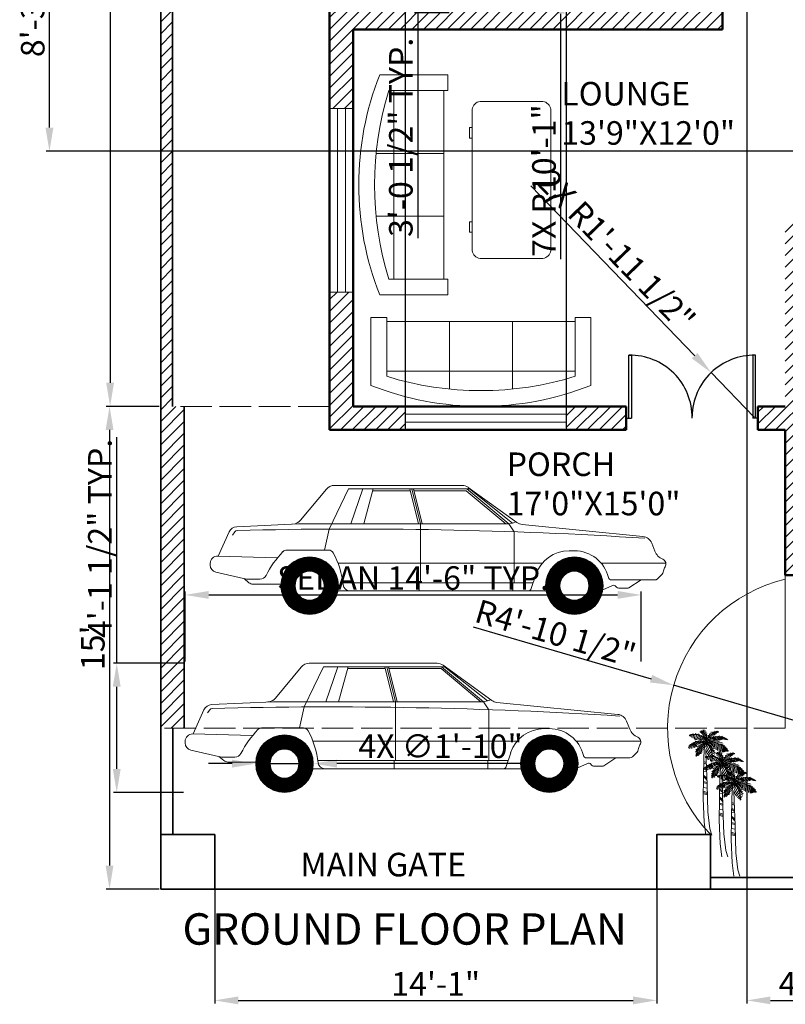
# Model space of a CAD drawing. Units: inches. Extents: x 36184 to 36805, y 18177 to 19069.
# Tile 1 of 5: x 36191 to 36484, y 18183 to 18560. Entities that reach past the tile are written whole.
import ezdxf

# ---------------------------------------------------------------- set-up
doc = ezdxf.new("R2010")
doc.units = ezdxf.units.IN
doc.linetypes.add('ACAD_ISO02W100', pattern=[15, 12, -3])
for name, color, linetype, lineweight in [('A-ANNO-DIMS', 2, 'Continuous', 18), ('A-ANNO-TEXT', 7, 'Continuous', 18), ('A-AREA-IDEN', 7, 'Continuous', 25), ('A-DOOR', 4, 'Continuous', 25), ('A-FURN', 8, 'Continuous', 18), ('A-GLAZ', 4, 'Continuous', 18), ('A-ROOF-OVHD', 8, 'ACAD_ISO02W100', 18), ('A-WALL', 7, 'Continuous', 50), ('C-PRKG-VEHS', 8, 'Continuous', 13), ('C-PROP', 7, 'Continuous', 35), ('L-HRDS', 8, 'Continuous', 18), ('L-PLNT', 94, 'Continuous', 13), ('L-SITE-GATE', 7, 'Continuous', 35), ('L-SITE-WALL', 7, 'Continuous', 35), ('L-WALL-PATT', 7, 'Continuous', 13)]:
    doc.layers.add(name, color=color, linetype=linetype, lineweight=lineweight)
doc.layers.add('A-WALL-PATT', color=244, linetype='Continuous', lineweight=13, true_color=0x991b1e)
doc.styles.get("Standard").update_dxf_attribs({"font": 'arial.ttf'})
doc.dimstyles.new('ISO-25', dxfattribs={"dimtxt": 9, "dimasz": 9, "dimexe": 1.25, "dimexo": 0.625, "dimtad": 1, "dimdec": 1, "dimrnd": 9, "dimlunit": 3, "dimtxsty": 'Standard', "dimcen": 2.5, "dimadec": 0, "dimazin": 0, "dimtfac": 1, "dimtdec": 1, "dimtmove": 0, "dimatfit": 3, "dimfxl": 1, "dimarcsym": 0})

# ---------------------------------------------------------------- blocks, each defined once
blk = doc.blocks.new('Car - sedan  side')
for p, q in [((-77.81, 49.34), (-126.58, 49.34)), ((-139.53, 35.99), (-129.64, 47.91)), ((-128.57, 32.64), (-121.22, 48.02)), ((-74.7, 48.02), (-121.22, 48.02)), ((-120.32, 34.67), (-115.67, 48.02)), ((-115.4, 34.67), (-111.74, 48.02)), ((-97.55, 47.3), (-111.94, 47.3)), ((-94.41, 34.67), (-97.73, 48.02)), ((-93.72, 34.67), (-97.04, 48.02)), ((-93.03, 34.67), (-96.34, 48.02)), ((-76.26, 47.3), (-96.16, 47.3)), ((-61.08, 34.66), (-76.26, 47.3)), ((-60.02, 34.65), (-76.07, 48.02)), ((-56.87, 35.13), (-75.48, 48.59)), ((-58.54, 34.93), (-74.99, 48.02)), ((-140.23, 34.67), (-163.88, 33.56)), ((-62.28, 34.67), (-140.23, 34.67)), ((-93.72, 19.62), (-93.72, 34.67)), ((-62.28, 34.67), (-60.02, 34.65)), ((-60.02, 34.65), (-58.54, 34.93)), ((-57.97, 31.61), (-60.02, 34.65)), ((-57.21, 35.38), (-58.54, 34.93)), ((-54.93, 34.4), (-8.75, 29.8)), ((-170.93, 22.32), (-166.81, 31.56)), ((-164.57, 31.6), (-165.48, 30.35)), ((-130.39, 24.63), (-128.57, 32.64)), ((-57.97, 19.62), (-57.97, 31.61)), ((-4.21, 24.18), (-5.42, 27.27)), ((-128.78, 24.63), (-144.79, 24.63)), ((-36.97, 24.38), (-34.94, 24.38)), ((-174, 19.51), (-174, 18.91)), ((-148.26, 21.7), (-171.11, 22.33)), ((-47.2, 19.62), (-125.23, 19.62)), ((-93.72, 12.14), (-93.72, 19.62)), ((-57.97, 12.14), (-57.97, 19.62)), ((0, 19.62), (-24.7, 19.62)), ((-160.12, 13.48), (-171.81, 16.16)), ((-51.4, 9.89), (-49.69, 15.14)), ((-159.22, 12.14), (-161.08, 13.7)), ((-155.01, 13.48), (-160.12, 13.48)), ((-147.03, 11.6), (-157.73, 11.6)), ((-50.67, 12.14), (-123.32, 12.14)), ((-94.21, 9.03), (-94.21, 12.14)), ((-58.39, 9.03), (-58.39, 12.14)), ((-4.23, 13.19), (-20.72, 13.19)), ((-9.5, 13.19), (-14.1, 10.2)), ((-3.22, 13.59), (-1.77, 14.97)), ((-120.62, 9.03), (-125.23, 9.03)), ((-45.76, 9.03), (-120.62, 9.03)), ((-20.36, 11.06), (-24.06, 9.44)), ((-18.83, 10.42), (-19.11, 10.76)), ((-14.68, 10.03), (-18.01, 10.03))]:
    blk.add_line(p, q)
at = {"const_width": 5.49}
for points in [[(-127.8, 11, -1), (-144.3, 11, -1)], [(-26.69, 11, -1), (-43.19, 11, -1)]]:
    blk.add_lwpolyline(points, format="xyb", close=True, dxfattribs=at)
for centre, radius in [((-136.05, 11), 11), ((-34.94, 11), 11), ((-136.05, 11), 5.51), ((-34.94, 11), 5.51)]:
    blk.add_circle(centre, radius)
for centre, radius, start, end in [((-126.58, 45.38), 3.97, 90, 140.3029), ((-77.81, 45.38), 3.97, 54.135, 90), ((-142.58, 38.53), 3.97, 272.6827, 320.3029), ((-54.54, 38.35), 3.97, 234.135, 264.3123), ((-163.72, 30.18), 3.38, 92.6827, 155.9736), ((-163.62, 30.91), 1.17, 91.491, 143.9553), ((-118.51, -1702.12), 1734.79, 86.34698, 91.49105), ((-9.15, 25.82), 4, 21.3107, 84.3123), ((-118.09, -2.78), 38.85, 136.3964, 152.9097), ((-144.79, 22.64), 1.98, 90, 136.3964), ((-128.78, 22.64), 1.98, 28.1371, 90), ((-157.14, 7.48), 34.14, 6.5135, 28.1371), ((-36.97, 11), 13.38, 90, 161.9732), ((-34.94, 11), 13.38, 13.5864, 90), ((0.9, 26.18), 5.49, 201.3107, 247.7048), ((-171.18, 19.51), 2.82, 88.4193, 180), ((-171.18, 18.91), 2.82, 180, 257.0905), ((-1.92, 19.3), 1.94, 325.3744, 67.7048), ((-3.82, 17.12), 2.96, 313.7173, 352.3839), ((2.46, 16.28), 3.37, 145.3744, 172.3839), ((-157.73, 13.93), 2.32, 230.1291, 270), ((-155.01, 16.1), 2.62, 270, 332.9097), ((-120.62, 11.65), 2.62, 186.5135, 270), ((-20.72, 14.43), 1.24, 193.5864, 270), ((-4.23, 14.65), 1.46, 270, 313.7173), ((-52.58, 10.27), 1.24, 270, 341.9732), ((-19.93, 10.09), 1.06, 39.301, 113.7159), ((-18.01, 11.09), 1.06, 219.301, 270), ((-14.68, 11.09), 1.06, 270, 303.047)]:
    blk.add_arc(centre, radius, start, end)
blk = doc.blocks.new('Tree - palm elevation')
for p, q in [((-29.729, 190.759), (-31.469, 191.255)), ((-30.309, 190.512), (-30.695, 189.025)), ((-25.283, 191.751), (-29.342, 192.246)), ((-28.763, 190.759), (-28.763, 188.281)), ((-26.443, 191.503), (-26.636, 186.051)), ((-20.064, 191.751), (-25.863, 193.238)), ((-23.737, 191.751), (-24.51, 185.06)), ((-21.031, 191.998), (-21.804, 183.325)), ((-15.232, 191.255), (-20.644, 193.981)), ((-17.551, 191.503), (-20.451, 181.343)), ((-14.265, 190.759), (-18.131, 182.086)), ((-9.433, 189.025), (-15.618, 193.238)), ((-11.753, 189.768), (-15.425, 182.83)), ((-6.727, 197.202), (-11.366, 197.45)), ((-3.441, 194.477), (-10.013, 195.716)), ((-1.894, 192.494), (-9.24, 193.733)), ((-6.147, 186.299), (-9.24, 190.264)), ((-7.5, 199.68), (-7.5, 197.946)), ((-0.541, 189.52), (-7.307, 192.494)), ((-5.76, 190.016), (0.618, 185.308)), ((-5.567, 196.707), (-4.987, 201.167)), ((-4.407, 195.716), (-3.247, 200.672)), ((-2.474, 193.733), (-1.315, 199.433)), ((-1.121, 190.759), (0.232, 196.955)), ((0.038, 188.281), (1.778, 193.981)), ((1.005, 185.803), (2.358, 190.759)), ((4.098, 185.06), (4.678, 190.512)), ((5.837, 187.786), (7.577, 194.229)), ((6.997, 188.529), (12.216, 187.786)), ((8.544, 190.512), (13.763, 189.52)), ((9.317, 191.255), (10.283, 196.955)), ((11.25, 192.494), (15.889, 190.512)), ((11.829, 192.99), (13.182, 197.45)), ((13.956, 194.229), (14.729, 196.955)), ((14.536, 193.981), (17.242, 191.255)), ((15.116, 194.477), (17.822, 198.689)), ((15.695, 186.299), (19.368, 188.777)), ((16.082, 194.972), (17.822, 192.494)), ((18.015, 195.716), (20.914, 198.689)), ((18.015, 195.468), (18.981, 192.494)), ((19.368, 196.459), (19.948, 193.733)), ((19.368, 187.29), (26.133, 189.768)), ((20.914, 196.459), (21.301, 194.972)), ((21.301, 196.459), (22.847, 198.441)), ((22.074, 196.707), (23.427, 195.716)), ((23.234, 196.707), (23.62, 197.698)), ((24.78, 187.538), (31.546, 188.777)), ((-28.956, 172.174), (-32.435, 170.192)), ((-31.082, 169.944), (-32.435, 169.2)), ((-27.409, 173.413), (-30.695, 172.67)), ((-29.922, 170.687), (-27.989, 165.235)), ((-25.09, 175.148), (-28.376, 174.404)), ((-27.989, 172.422), (-26.056, 166.227)), ((-26.829, 173.661), (-23.544, 167.218)), ((-25.476, 174.652), (-21.224, 167.466)), ((-21.031, 177.626), (-24.897, 176.387)), ((-24.317, 175.891), (-18.711, 168.457)), ((-22.191, 176.635), (-16.391, 169.448)), ((-15.618, 179.36), (-20.644, 178.617)), ((-20.064, 177.626), (-15.812, 172.67)), ((-17.358, 178.617), (-13.299, 173.661)), ((-8.466, 171.678), (-16.585, 167.713)), ((-15.038, 179.36), (-10.786, 174.404)), ((-4.214, 175.148), (-14.072, 170.935)), ((-8.08, 188.034), (-12.912, 182.83)), ((-12.332, 180.104), (-9.433, 175.643)), ((-4.987, 185.803), (-10.979, 182.086)), ((-10.206, 180.104), (-8.08, 175.891)), ((-8.853, 170.935), (-7.113, 160.527)), ((-1.701, 176.882), (-8.66, 175.396)), ((-8.273, 180.104), (-6.147, 176.635)), ((-3.247, 183.821), (-8.08, 181.838)), ((-6.92, 172.917), (-5.374, 163.253)), ((-6.34, 179.608), (-4.6, 177.13)), ((-5.76, 188.034), (-1.508, 182.582)), ((-1.315, 181.591), (-5.374, 181.095)), ((-4.6, 174.9), (-4.021, 166.722)), ((-4.021, 179.36), (-2.861, 177.378)), ((-2.668, 185.803), (1.198, 181.343)), ((-2.668, 176.387), (-2.376, 170.594)), ((-0.348, 180.352), (-1.894, 180.104)), ((-0.928, 176.882), (-1.508, 173.909)), ((2.551, 175.891), (-0.928, 171.431)), ((3.711, 174.404), (-0.541, 167.961)), ((5.257, 171.926), (-0.155, 163.005)), ((1.585, 177.13), (0.038, 174.652)), ((1.005, 182.582), (2.938, 186.547)), ((1.585, 177.13), (6.61, 176.139)), ((2.938, 182.582), (6.61, 183.821)), ((2.938, 175.891), (8.737, 173.413)), ((4.098, 180.847), (8.35, 179.608)), ((4.291, 173.909), (12.216, 168.953)), ((4.871, 186.051), (10.09, 186.547)), ((4.871, 181.591), (8.544, 184.812)), ((5.644, 181.838), (13.569, 178.865)), ((6.224, 178.121), (8.157, 175.148)), ((6.417, 170.439), (14.729, 164.492)), ((7.384, 178.369), (10.476, 179.36)), ((7.77, 183.325), (16.082, 179.856)), ((8.157, 178.121), (10.476, 172.422)), ((9.51, 184.317), (15.502, 188.034)), ((10.476, 177.874), (12.796, 169.696)), ((11.25, 184.812), (17.628, 180.352)), ((11.829, 177.874), (18.015, 179.113)), ((13.182, 177.874), (14.729, 166.97)), ((14.536, 185.803), (19.948, 180.847)), ((15.889, 177.13), (16.855, 164.492)), ((17.242, 186.547), (23.041, 180.599)), ((18.015, 177.13), (26.133, 179.113)), ((18.981, 175.891), (19.561, 163.005)), ((20.721, 187.042), (25.167, 181.343)), ((20.914, 175.891), (30.966, 176.635)), ((21.688, 175.396), (22.074, 161.518)), ((23.814, 187.29), (26.907, 181.343)), ((23.814, 174.404), (25.554, 160.279)), ((25.554, 173.661), (33.285, 173.661)), ((26.133, 187.29), (29.419, 181.838)), ((26.52, 173.165), (28.066, 159.784)), ((28.066, 187.29), (30.966, 182.582)), ((28.839, 172.174), (36.378, 170.687)), ((29.226, 171.926), (30.966, 158.545)), ((29.806, 186.795), (32.319, 183.078)), ((29.999, 186.795), (33.092, 187.29)), ((30.966, 170.687), (38.891, 167.713)), ((32.126, 169.696), (32.512, 158.545)), ((32.512, 186.299), (35.218, 186.299)), ((33.479, 186.051), (34.445, 182.83)), ((35.605, 185.556), (37.151, 185.308)), ((35.798, 185.308), (36.958, 181.591)), ((38.118, 184.317), (38.504, 181.838)), ((39.857, 182.83), (40.244, 181.591)), ((-32.628, 167.961), (-33.208, 167.961)), ((-32.628, 167.713), (-32.435, 165.979)), ((-31.662, 168.705), (-31.082, 165.483)), ((-14.265, 164.244), (-19.678, 158.049)), ((-16.005, 160.031), (-19.484, 154.084)), ((-18.131, 153.589), (-19.484, 151.606)), ((-12.139, 167.961), (-19.098, 162.014)), ((-17.938, 152.597), (-16.972, 151.111)), ((-17.358, 155.819), (-14.845, 151.358)), ((-16.585, 158.545), (-13.106, 152.35)), ((-15.618, 160.775), (-12.332, 154.332)), ((-14.265, 163.749), (-10.786, 154.828)), ((-12.719, 166.722), (-9.046, 154.828)), ((-10.979, 168.457), (-7.887, 157.801)), ((7.384, 168.705), (0.812, 157.553)), ((9.317, 164.244), (2.358, 154.332)), ((10.863, 159.784), (4.484, 152.35)), ((11.829, 155.075), (6.804, 150.119)), ((8.544, 165.979), (16.662, 160.527)), ((12.603, 151.111), (8.544, 148.385)), ((10.09, 162.51), (17.435, 157.058)), ((11.443, 157.553), (16.855, 154.332)), ((12.216, 153.093), (16.082, 151.606)), ((34.058, 168.705), (34.445, 158.545)), ((35.412, 167.713), (41.404, 164.988)), ((36.378, 166.474), (35.605, 158.792)), ((37.731, 165.235), (36.958, 159.288)), ((37.924, 165.235), (41.404, 163.749)), ((38.504, 164.492), (38.504, 159.536)), ((39.664, 163.253), (42.37, 161.766)), ((39.857, 162.757), (39.857, 160.031)), ((40.824, 161.766), (41.21, 160.031)), ((41.21, 161.518), (42.757, 160.279)), ((-4.081, 140.645), (0.753, 138.261)), ((-4.081, 137.547), (0.753, 135.163)), ((12.216, 148.137), (10.09, 147.393)), ((12.409, 145.659), (11.056, 145.659)), ((12.409, 146.898), (13.763, 146.402)), ((12.603, 149.872), (15.116, 149.128)), ((-4.267, 114.428), (1.682, 108.708)), ((-4.081, 129.205), (1.124, 126.821)), ((-4.081, 127.298), (1.31, 123.246)), ((-4.081, 121.578), (1.31, 120.863)), ((-4.639, 102.273), (1.868, 100.604)), ((-4.453, 112.283), (1.682, 105.133)), ((-4.453, 99.651), (2.24, 98.459)), ((-4.825, 83.921), (2.612, 81.061)), ((-4.639, 81.299), (2.797, 78.916)), ((-4.639, 78.916), (2.797, 76.771)), ((-4.453, 91.071), (2.426, 89.641))]:
    blk.add_line(p, q)
for points in [[(-2.363, 170.553), (-3.88, 148.505), (-4.988, 69.634), (-3.325, 24.869), (0, 0)], [(-0.116, 162.848), (0.554, 143.532), (2.217, 96.635), (3.88, 44.054), (7.76, 12.079), (11.64, 0)]]:
    blk.add_lwpolyline(points)
for centre, radius, start, end in [((-21.738, 166.094), 25.899, 27.67115, 112.5305), ((-18.427, 181.448), 19.715, 350.285, 64.11229), ((25.595, 171.567), 25.395, 91.40319, 163.882), ((-9.259, 151.732), 28.386, 68.38311, 147.5322), ((14.394, 148.393), 32.752, 113.7592, 177.4133), ((23.687, 155.341), 32.188, 56.19272, 134.3213), ((5.828, 132.718), 45.639, 35.98777, 95.82273), ((-32.8, 147.923), 45.309, 356.1943, 41.37848)]:
    blk.add_arc(centre, radius, start, end)
blk = doc.blocks.new('Sofa - Roundback 7 ft.')
for p, q in [((-12.00002, -32.4421), (-12.00003, -6.5971)), ((11.99997, -32.4421), (11.99998, -6.5971)), ((-36.000027, -34), (-36.000027, -11.4696)), ((-35.999844, -13.3819), (35.9998, -13.3819)), ((35.99998, -34), (35.99998, -11.4696)), ((-36.000027, -32.4421), (35.99998, -32.4421))]:
    blk.add_line(p, q)
for points in [[(-36.000027, -34), (-42.000027, -34), (-42.000027, -8)], [(41.99998, -8), (41.99998, -34), (35.99998, -34)]]:
    blk.add_lwpolyline(points)
for centre, radius, start, end in [((0, -114.25), 114.25, 68.43141, 111.5686), ((-0.00001, -127.1968), 121.1968, 72.72033, 107.2797)]:
    blk.add_arc(centre, radius, start, end)
blk = doc.blocks.new('Desk - 30 x 60 in.')
for p, q in [((-26.999995, 0), (26.999995, 0)), ((-29.999995, -27), (-29.999995, -3)), ((29.999995, -3), (29.999995, -27)), ((26.999995, -30), (-26.999995, -30)), ((-20.000005, -30), (-20.000005, -31)), ((-16.000005, -31), (-16.000005, -30)), ((15.999995, -31), (15.999995, -30)), ((19.999995, -30), (19.999995, -31)), ((-20.000005, -31), (-16.000005, -31)), ((19.999995, -31), (15.999995, -31))]:
    blk.add_line(p, q)
for centre, start, end in [((-26.499995, -3.5), 98.1301, 171.8699), ((26.499995, -3.5), 8.130102, 81.8699), ((-26.499995, -26.5), 188.1301, 261.8699), ((26.499995, -26.5), 278.1301, 351.8699)]:
    blk.add_arc(centre, 3.535534, start, end)
blk = doc.blocks.new('*D14')
at = {"layer": 'A-ANNO-DIMS', "color": 0, "lineweight": -2, "transparency": 16777216}
for p, q in [((36244.69, 19007.3), (36224.73, 19007.3)), ((36225.98, 18998.3), (36225.98, 18420.79)), ((36244.69, 18411.79), (36224.73, 18411.79))]:
    blk.add_line(p, q, dxfattribs=at)
at = {"layer": 'A-ANNO-DIMS', "color": 0, "transparency": 16777216}
for points in [[(36224.48, 18998.3), (36227.48, 18998.3), (36225.98, 19007.3)], [(36224.48, 18420.79), (36227.48, 18420.79), (36225.98, 18411.79)]]:
    blk.add_solid(points, dxfattribs=at)
at = {"layer": 'Defpoints', "color": 0, "transparency": 16777216}
for p in [(36245.31, 19007.3), (36225.98, 18411.79), (36245.31, 18411.79)]:
    blk.add_point(p, dxfattribs=at)
at = {"layer": 'A-ANNO-DIMS', "color": 0, "transparency": 16777216, "insert": (36220.76, 18709.54), "char_height": 9, "attachment_point": 5, "rotation": 90}
blk.add_mtext('49\'-6"', dxfattribs=at)
blk = doc.blocks.new('*D16')
at = {"layer": 'A-ANNO-DIMS', "color": 0, "lineweight": -2, "transparency": 16777216}
for p, q in [((36244.69, 18411.79), (36224.51, 18411.79)), ((36225.76, 18402.79), (36225.76, 18236.3)), ((36244.69, 18227.3), (36224.51, 18227.3))]:
    blk.add_line(p, q, dxfattribs=at)
at = {"layer": 'A-ANNO-DIMS', "color": 0, "transparency": 16777216}
for points in [[(36224.26, 18402.79), (36227.26, 18402.79), (36225.76, 18411.79)], [(36224.26, 18236.3), (36227.26, 18236.3), (36225.76, 18227.3)]]:
    blk.add_solid(points, dxfattribs=at)
at = {"layer": 'Defpoints', "color": 0, "transparency": 16777216}
for p in [(36245.31, 18411.79), (36225.76, 18227.3), (36245.31, 18227.3)]:
    blk.add_point(p, dxfattribs=at)
at = {"layer": 'A-ANNO-DIMS', "color": 0, "transparency": 16777216, "insert": (36220.54, 18319.54), "char_height": 9, "attachment_point": 5, "rotation": 90}
blk.add_mtext("15'", dxfattribs=at)
blk = doc.blocks.new('DOOR-LEAF-24IN')
for p, q in [((1, 0), (1, 24)), ((1, 24), (2, 24)), ((2, 24), (2, 0)), ((0, 0), (1, 0)), ((1, 0), (2, 0))]:
    blk.add_line(p, q)
blk = doc.blocks.new('*D23')
at = {"layer": 'A-ANNO-DIMS', "color": 0, "lineweight": -2, "transparency": 16777216}
for p, q in [((36355.41, 18598.8), (36342.19, 18598.8)), ((36343.44, 18589.8), (36343.44, 18571.14)), ((36355.41, 18562.14), (36342.19, 18562.14)), ((36343.44, 18562.14), (36343.44, 18476.06))]:
    blk.add_line(p, q, dxfattribs=at)
at = {"layer": 'A-ANNO-DIMS', "color": 0, "transparency": 16777216}
for points in [[(36341.94, 18589.8), (36344.94, 18589.8), (36343.44, 18598.8)], [(36341.94, 18571.14), (36344.94, 18571.14), (36343.44, 18562.14)]]:
    blk.add_solid(points, dxfattribs=at)
at = {"layer": 'Defpoints', "color": 0, "transparency": 16777216}
for p in [(36356.04, 18598.8), (36343.44, 18562.14), (36356.04, 18562.14)]:
    blk.add_point(p, dxfattribs=at)
at = {"layer": 'A-ANNO-DIMS', "color": 0, "transparency": 16777216, "insert": (36338.16, 18514.6), "char_height": 9, "attachment_point": 5, "rotation": 90}
blk.add_mtext('3\'-0 1/2" TYP.', dxfattribs=at)
blk = doc.blocks.new('*D36')
at = {"layer": 'A-ANNO-DIMS', "color": 0, "lineweight": -2, "transparency": 16777216}
for p, q in [((36254.63, 18314.25), (36254.63, 18340.99)), ((36263.63, 18339.74), (36419.74, 18339.74)), ((36428.74, 18314.25), (36428.74, 18340.99))]:
    blk.add_line(p, q, dxfattribs=at)
at = {"layer": 'A-ANNO-DIMS', "color": 0, "transparency": 16777216}
for points in [[(36263.63, 18341.24), (36263.63, 18338.24), (36254.63, 18339.74)], [(36419.74, 18341.24), (36419.74, 18338.24), (36428.74, 18339.74)]]:
    blk.add_solid(points, dxfattribs=at)
at = {"layer": 'Defpoints', "color": 0, "transparency": 16777216}
for p in [(36428.74, 18339.74), (36254.63, 18313.62), (36428.74, 18313.62)]:
    blk.add_point(p, dxfattribs=at)
at = {"layer": 'A-ANNO-DIMS', "color": 0, "transparency": 16777216, "insert": (36341.68, 18345.02), "char_height": 9, "attachment_point": 5}
blk.add_mtext('SEDAN 14\'-6" TYP.', dxfattribs=at)
blk = doc.blocks.new('*D37')
at = {"layer": 'A-ANNO-DIMS', "color": 0, "lineweight": -2, "transparency": 16777216}
for p, q in [((36228.51, 18313.62), (36228.51, 18400.07)), ((36254, 18313.62), (36227.26, 18313.62)), ((36228.51, 18273.28), (36228.51, 18304.62)), ((36254, 18264.28), (36227.26, 18264.28))]:
    blk.add_line(p, q, dxfattribs=at)
at = {"layer": 'A-ANNO-DIMS', "color": 0, "transparency": 16777216}
for points in [[(36227.01, 18304.62), (36230.01, 18304.62), (36228.51, 18313.62)], [(36227.01, 18273.28), (36230.01, 18273.28), (36228.51, 18264.28)]]:
    blk.add_solid(points, dxfattribs=at)
at = {"layer": 'Defpoints', "color": 0, "transparency": 16777216}
for p in [(36228.51, 18313.62), (36254.63, 18313.62), (36254.63, 18264.28)]:
    blk.add_point(p, dxfattribs=at)
at = {"layer": 'A-ANNO-DIMS', "color": 0, "transparency": 16777216, "insert": (36223.23, 18361.34), "char_height": 9, "attachment_point": 5, "rotation": 90}
blk.add_mtext('4\'-1 1/2" TYP.', dxfattribs=at)
blk = doc.blocks.new('*D44')
at = {"layer": 'A-ANNO-DIMS', "color": 0, "lineweight": -2, "transparency": 16777216}
for p, q in [((36265.92, 18247.5), (36265.92, 18183.55)), ((36434.7, 18247.5), (36434.7, 18183.55)), ((36274.92, 18184.8), (36425.7, 18184.8))]:
    blk.add_line(p, q, dxfattribs=at)
at = {"layer": 'A-ANNO-DIMS', "color": 0, "transparency": 16777216}
for points in [[(36274.92, 18186.3), (36274.92, 18183.3), (36265.92, 18184.8)], [(36425.7, 18186.3), (36425.7, 18183.3), (36434.7, 18184.8)]]:
    blk.add_solid(points, dxfattribs=at)
at = {"layer": 'Defpoints', "color": 0, "transparency": 16777216}
for p in [(36265.92, 18248.13), (36434.7, 18248.13), (36434.7, 18184.8)]:
    blk.add_point(p, dxfattribs=at)
at = {"layer": 'A-ANNO-DIMS', "color": 0, "transparency": 16777216, "insert": (36350.31, 18189.95), "char_height": 9, "attachment_point": 5}
blk.add_mtext('14\'-1"', dxfattribs=at)
blk = doc.blocks.new('*D47')
at = {"layer": 'A-ANNO-DIMS', "color": 0, "lineweight": -2, "transparency": 16777216}
for p, q in [((36519.19, 18608.3), (36201.56, 18608.3)), ((36202.81, 18518.3), (36202.81, 18599.3)), ((36519.19, 18509.3), (36201.56, 18509.3))]:
    blk.add_line(p, q, dxfattribs=at)
at = {"layer": 'A-ANNO-DIMS', "color": 0, "transparency": 16777216}
for points in [[(36201.31, 18599.3), (36204.31, 18599.3), (36202.81, 18608.3)], [(36201.31, 18518.3), (36204.31, 18518.3), (36202.81, 18509.3)]]:
    blk.add_solid(points, dxfattribs=at)
at = {"layer": 'Defpoints', "color": 0, "transparency": 16777216}
for p in [(36202.81, 18608.3), (36519.81, 18608.3), (36519.81, 18509.3)]:
    blk.add_point(p, dxfattribs=at)
at = {"layer": 'A-ANNO-DIMS', "color": 0, "transparency": 16777216, "insert": (36197.59, 18558.8), "char_height": 9, "attachment_point": 5, "rotation": 90}
blk.add_mtext('8\'-3"', dxfattribs=at)
blk = doc.blocks.new('*D59')
at = {"layer": 'A-ANNO-DIMS', "color": 0, "lineweight": -2, "transparency": 16777216}
for p, q in [((36469.15, 18918.18), (36469.15, 18183.55)), ((36527.35, 18918.18), (36527.35, 18183.55)), ((36478.15, 18184.8), (36518.35, 18184.8))]:
    blk.add_line(p, q, dxfattribs=at)
at = {"layer": 'A-ANNO-DIMS', "color": 0, "transparency": 16777216}
for points in [[(36478.15, 18186.3), (36478.15, 18183.3), (36469.15, 18184.8)], [(36518.35, 18186.3), (36518.35, 18183.3), (36527.35, 18184.8)]]:
    blk.add_solid(points, dxfattribs=at)
at = {"layer": 'Defpoints', "color": 0, "transparency": 16777216}
for p in [(36469.15, 18918.8), (36527.35, 18918.8), (36527.35, 18184.8)]:
    blk.add_point(p, dxfattribs=at)
at = {"layer": 'A-ANNO-DIMS', "color": 0, "transparency": 16777216, "insert": (36498.25, 18190.02), "char_height": 9, "attachment_point": 5}
blk.add_mtext('4\'-10"', dxfattribs=at)
blk = doc.blocks.new('*D60')
at = {"layer": 'A-ANNO-DIMS', "color": 0, "lineweight": -2, "transparency": 16777216}
for p, q in [((36338.76, 18403.43), (36338.76, 19051.05)), ((36347.76, 19049.8), (36391.25, 19049.8)), ((36400.25, 18403.43), (36400.25, 19051.05))]:
    blk.add_line(p, q, dxfattribs=at)
at = {"layer": 'A-ANNO-DIMS', "color": 0, "transparency": 16777216}
for points in [[(36347.76, 19051.3), (36347.76, 19048.3), (36338.76, 19049.8)], [(36391.25, 19051.3), (36391.25, 19048.3), (36400.25, 19049.8)]]:
    blk.add_solid(points, dxfattribs=at)
at = {"layer": 'Defpoints', "color": 0, "transparency": 16777216}
for p in [(36400.25, 19049.8), (36338.76, 18402.8), (36400.25, 18402.8)]:
    blk.add_point(p, dxfattribs=at)
at = {"layer": 'A-ANNO-DIMS', "color": 0, "transparency": 16777216, "insert": (36369.51, 19055.08), "char_height": 9, "attachment_point": 5}
blk.add_mtext('5\'-1 1/2"', dxfattribs=at)
blk = doc.blocks.new('*D61')
at = {"layer": 'A-ANNO-DIMS', "color": 0, "lineweight": -2, "transparency": 16777216}
for p, q in [((36364.63, 18327.57), (36432.54, 18307.73)), ((36497.33, 18288.82), (36441.18, 18305.21))]:
    blk.add_line(p, q, dxfattribs=at)
at = {"layer": 'A-ANNO-DIMS', "color": 0, "transparency": 16777216}
blk.add_solid([(36432.97, 18309.17), (36432.12, 18306.29), (36441.18, 18305.21)], dxfattribs=at)
at = {"layer": 'Defpoints', "color": 0, "transparency": 16777216}
for p in [(36441.18, 18305.21), (36497.33, 18288.82)]:
    blk.add_point(p, dxfattribs=at)
at = {"layer": 'A-ANNO-DIMS', "color": 0, "transparency": 16777216, "insert": (36395.75, 18323.98), "char_height": 9, "attachment_point": 5, "rotation": 343.7204}
blk.add_mtext('R4\'-10 1/2"', dxfattribs=at)
blk = doc.blocks.new('*D67')
at = {"layer": 'A-ANNO-DIMS', "color": 0, "lineweight": -2, "transparency": 16777216}
for p, q in [((36386.58, 18496.12), (36449.22, 18431.16)), ((36471.88, 18407.66), (36455.47, 18424.68))]:
    blk.add_line(p, q, dxfattribs=at)
at = {"layer": 'A-ANNO-DIMS', "color": 0, "transparency": 16777216}
blk.add_solid([(36450.3, 18432.2), (36448.14, 18430.12), (36455.47, 18424.68)], dxfattribs=at)
at = {"layer": 'Defpoints', "color": 0, "transparency": 16777216}
for p in [(36455.47, 18424.68), (36471.88, 18407.66)]:
    blk.add_point(p, dxfattribs=at)
at = {"layer": 'A-ANNO-DIMS', "color": 0, "transparency": 16777216, "insert": (36418.57, 18470.54), "char_height": 9, "attachment_point": 5, "rotation": 313.9601}
blk.add_mtext('2X R1\'-11 1/2"', dxfattribs=at)
blk = doc.blocks.new('*D70')
at = {"layer": 'A-ANNO-DIMS', "color": 0, "lineweight": -2, "transparency": 16777216}
for p, q in [((36398.04, 18692), (36398.04, 18570.8)), ((36398.04, 18468.06), (36398.04, 18561.8))]:
    blk.add_line(p, q, dxfattribs=at)
at = {"layer": 'A-ANNO-DIMS', "color": 0, "transparency": 16777216}
blk.add_solid([(36396.54, 18561.8), (36399.54, 18561.8), (36398.04, 18570.8)], dxfattribs=at)
at = {"layer": 'Defpoints', "color": 0, "transparency": 16777216}
for p in [(36398.04, 18692), (36398.04, 18570.8)]:
    blk.add_point(p, dxfattribs=at)
at = {"layer": 'A-ANNO-DIMS', "color": 0, "transparency": 16777216, "insert": (36392.82, 18498.08), "char_height": 9, "attachment_point": 5, "rotation": 89.9998}
blk.add_mtext('7X R10\'-1"', dxfattribs=at)
blk = doc.blocks.new('*D72')
at = {"layer": 'A-ANNO-DIMS', "color": 0, "lineweight": -2, "transparency": 16777216}
for p, q in [((36272.58, 18275.27), (36263.58, 18275.27)), ((36281.58, 18275.27), (36303.58, 18275.27)), ((36382.76, 18275.27), (36312.58, 18275.27))]:
    blk.add_line(p, q, dxfattribs=at)
at = {"layer": 'A-ANNO-DIMS', "color": 0, "transparency": 16777216}
for points in [[(36272.58, 18276.77), (36272.58, 18273.77), (36281.58, 18275.27)], [(36312.58, 18276.77), (36312.58, 18273.77), (36303.58, 18275.27)]]:
    blk.add_solid(points, dxfattribs=at)
at = {"layer": 'Defpoints', "color": 0, "transparency": 16777216}
for p in [(36281.58, 18275.27), (36303.58, 18275.27)]:
    blk.add_point(p, dxfattribs=at)
at = {"layer": 'A-ANNO-DIMS', "color": 0, "transparency": 16777216, "insert": (36352.17, 18280.75), "char_height": 9, "attachment_point": 5, "rotation": 0.0006}
blk.add_mtext('4X ∅1\'-10"', dxfattribs=at)

msp = doc.modelspace()

# ---------------------------------------------------------------- hatches: boundary and pattern name
at = {"layer": 'A-WALL-PATT'}
h = msp.add_hatch(dxfattribs=at)
h.set_pattern_fill('ANSI31', color=256)
h.paths.add_polyline_path([(36318.81, 18555.8), (36459.81, 18555.8), (36459.81, 18705.8), (36440.41, 18705.8), (36440.41, 18696.8), (36450.81, 18696.8), (36450.81, 18564.8), (36318.81, 18564.8), (36318.81, 18591.83), (36309.81, 18591.83), (36309.81, 18525.65), (36318.81, 18525.65)], flags=17)
h.paths.add_polyline_path([(36318.81, 18455.41), (36309.81, 18455.41), (36309.81, 18402.8), (36338.76, 18402.8), (36338.76, 18411.8), (36318.81, 18411.8)], flags=17)
h.paths.add_polyline_path([(36423.09, 18411.8), (36400.25, 18411.8), (36400.25, 18402.8), (36423.09, 18402.8)], flags=17)
h.paths.add_polyline_path([(36492.81, 18478.27), (36496.58, 18481.34), (36494.6, 18487.78), (36492.81, 18486.25), (36483.81, 18479.84), (36483.81, 18411.8), (36473.38, 18411.8), (36473.38, 18402.8), (36483.81, 18402.8), (36483.81, 18356.3), (36483.81, 18347.3), (36519.81, 18347.3), (36524.04, 18347.3), (36524.04, 18356.3), (36492.81, 18356.3)], flags=17)
h.paths.add_polyline_path([(36665.31, 18608.3), (36660.81, 18608.3), (36660.81, 18557.3), (36646.76, 18557.3), (36646.76, 18552.8), (36660.81, 18552.8), (36660.81, 18504.8), (36650.24, 18504.8), (36650.24, 18500.3), (36660.81, 18500.3), (36660.81, 18356.3), (36622.58, 18356.3), (36622.58, 18347.3), (36665.31, 18347.3)])
h.paths.add_polyline_path([(36608.31, 18509.3), (36519.81, 18509.3), (36513.55, 18503.95), (36517.84, 18498.69), (36519.81, 18500.3), (36608.31, 18500.3)])
h.paths.add_polyline_path([(36254.31, 18411.79), (36249.81, 18411.79), (36249.81, 19002.8), (36553.31, 19002.8), (36553.31, 19007.3), (36245.31, 19007.3), (36245.31, 18288.82), (36254.31, 18288.82)])
h.paths.add_polyline_path([(36342.97, 18918.8), (36309.81, 18918.8), (36309.81, 18747.12), (36314.31, 18747.12), (36314.31, 18765.8), (36384.81, 18765.8), (36384.81, 18701.3), (36350.57, 18701.3), (36350.57, 18696.8), (36396.53, 18696.8), (36396.53, 18705.8), (36389.31, 18705.8), (36389.31, 18761.3), (36393.31, 18761.3), (36393.31, 18770.3), (36384.81, 18770.3), (36318.81, 18770.3), (36318.81, 18909.8), (36342.97, 18909.8)], flags=17)
h.paths.add_polyline_path([(36469.15, 18918.8), (36403.35, 18918.8), (36403.35, 18909.8), (36434.31, 18909.8), (36434.31, 18770.3), (36431, 18770.3), (36431, 18761.3), (36449.29, 18761.3), (36449.29, 18770.3), (36443.31, 18770.3), (36443.31, 18909.8), (36469.15, 18909.8)], flags=17)
h.paths.add_polyline_path([(36557.81, 18953.44), (36553.31, 18953.44), (36553.31, 18918.8), (36527.35, 18918.8), (36527.35, 18909.8), (36553.31, 18909.8), (36562.16, 18909.8), (36562.16, 18914.3), (36557.81, 18914.3)])
h.paths.add_polyline_path([(36665.31, 19007.3), (36553.31, 19007.3), (36553.31, 19002.8), (36553.31, 18989.93), (36557.81, 18989.93), (36557.81, 19002.8), (36660.81, 19002.8), (36660.81, 18765.8), (36656.73, 18765.8), (36656.73, 18761.3), (36660.81, 18761.3), (36660.81, 18617.3), (36654.49, 18617.3), (36654.49, 18608.3), (36665.31, 18608.3)])
h.paths.add_polyline_path([(36600.81, 18890.3), (36596.31, 18890.3), (36596.31, 18770.3), (36487.63, 18770.3), (36487.63, 18761.3), (36519.81, 18761.3), (36519.81, 18756.26), (36528.81, 18756.26), (36528.81, 18761.3), (36634.81, 18761.3), (36634.81, 18765.8), (36600.81, 18765.8), (36600.81, 18825.8), (36660.81, 18825.8), (36660.81, 18830.3), (36600.81, 18830.3)])
h.paths.add_polyline_path([(36600.81, 18914.3), (36596.31, 18914.3), (36591.43, 18914.3), (36591.43, 18909.8), (36596.31, 18909.8), (36596.31, 18890.3), (36660.81, 18890.3), (36660.81, 18894.8), (36600.81, 18894.8)], flags=17)
h.paths.add_polyline_path([(36623.57, 18617.3), (36528.81, 18617.3), (36528.81, 18717.38), (36519.81, 18717.38), (36519.81, 18608.3), (36608.31, 18608.3), (36608.31, 18603.13), (36617.31, 18603.13), (36617.31, 18608.3), (36623.57, 18608.3)])
h.paths.add_polyline_path([(36602.02, 18898.95), (36663.11, 18898.95), (36663.11, 18913.37), (36602.02, 18913.37)], flags=25)
at = {"layer": 'L-WALL-PATT'}
h = msp.add_hatch(dxfattribs=at)
h.set_pattern_fill('AR-CONC', color=256, scale=100)
h.paths.add_polyline_path([(36265.92, 18248.13), (36245.31, 18248.13), (36245.31, 18227.3), (36265.92, 18227.3)])
h.paths.add_polyline_path([(36455.31, 18248.13), (36434.7, 18248.13), (36434.7, 18227.3), (36455.31, 18227.3)])

# ---------------------------------------------------------------- linework, layer by layer
at = {"layer": 'A-DOOR'}
for centre, start, end in [((36424.59, 18407.66), 359.1333, 91.2115), ((36471.88, 18407.66), 88.7885, 179.1333)]:
    msp.add_arc(centre, 23.65, start, end, dxfattribs=at)
at = {"layer": 'A-GLAZ'}
for p, q in [((36318.81, 18525.65), (36309.81, 18525.65)), ((36312.81, 18525.65), (36312.81, 18455.41)), ((36315.81, 18525.65), (36315.81, 18455.41)), ((36318.81, 18455.41), (36309.81, 18455.41)), ((36338.76, 18411.8), (36338.76, 18402.8)), ((36400.25, 18411.8), (36400.25, 18402.8)), ((36400.25, 18408.8), (36338.76, 18408.8)), ((36400.25, 18405.8), (36338.76, 18405.8))]:
    msp.add_line(p, q, dxfattribs=at)
at = {"layer": 'A-ROOF-OVHD'}
for p, q in [((36309.81, 18411.79), (36249.81, 18411.79)), ((36483.81, 18347.3), (36483.81, 18288.82)), ((36483.81, 18288.82), (36245.31, 18288.82))]:
    msp.add_line(p, q, dxfattribs=at)
at = {"layer": 'A-WALL'}
for p, q in [((36309.81, 18918.8), (36309.81, 18402.8)), ((36459.81, 18705.8), (36459.81, 18555.8)), ((36459.81, 18555.8), (36318.81, 18555.8)), ((36318.81, 18555.8), (36318.81, 18411.8)), ((36423.09, 18411.8), (36318.81, 18411.8)), ((36423.09, 18411.8), (36423.09, 18402.8)), ((36483.81, 18411.8), (36473.38, 18411.8)), ((36473.38, 18411.8), (36473.38, 18402.8)), ((36423.09, 18402.8), (36309.81, 18402.8)), ((36483.81, 18402.8), (36473.38, 18402.8)), ((36483.81, 18356.3), (36483.81, 18402.8)), ((36483.81, 18347.3), (36483.81, 18356.3)), ((36519.81, 18347.3), (36483.81, 18347.3))]:
    msp.add_line(p, q, dxfattribs=at)
at = {"layer": 'C-PROP'}
for p, q in [((36245.31, 19007.3), (36245.31, 18227.3)), ((36245.31, 18227.3), (36665.31, 18227.3))]:
    msp.add_line(p, q, dxfattribs=at)
at = {"layer": 'L-HRDS'}
msp.add_line((36483.81, 18345.72), (36483.81, 18288.82), dxfattribs=at)
msp.add_arc((36497.33, 18288.82), 58.49, 103.3591, 224.0818, dxfattribs=at)
at = {"layer": 'L-SITE-GATE'}
for points in [[(36245.31, 18227.3), (36265.92, 18227.3), (36265.92, 18248.13), (36245.31, 18248.13)], [(36434.7, 18227.3), (36455.31, 18227.3), (36455.31, 18248.13), (36434.7, 18248.13)]]:
    msp.add_lwpolyline(points, close=True, dxfattribs=at)
at = {"layer": 'L-SITE-WALL'}
for p, q in [((36249.81, 19002.8), (36249.81, 18411.79)), ((36254.31, 18411.79), (36254.31, 18288.82)), ((36249.98, 18288.82), (36249.98, 18248.13)), ((36455.31, 18231.8), (36455.31, 18227.3)), ((36455.31, 18231.8), (36660.81, 18231.8))]:
    msp.add_line(p, q, dxfattribs=at)

# ---------------------------------------------------------------- block references
at = {"layer": 'A-DOOR'}
msp.add_blockref('DOOR-LEAF-24IN', (36423.09, 18407.3), dxfattribs=at)
at = {"layer": 'A-DOOR', "extrusion": (0, 0, -1), "zscale": -1}
msp.add_blockref('DOOR-LEAF-24IN', (-36473.38, 18407.3), dxfattribs=at)
at = {"layer": 'A-FURN'}
for name, p, rotation in [('Sofa - Roundback 7 ft.', (36320.93, 18496.46), 89.99999999999999), ('Desk - 30 x 60 in.', (36394.23, 18498.32), 270), ('Sofa - Roundback 7 ft.', (36367.59, 18411.8), 180)]:
    msp.add_blockref(name, p, dxfattribs=dict(at, rotation=rotation))
at = {"layer": 'C-PRKG-VEHS'}
for p in [(36438.21, 18332.26), (36428.63, 18264.28)]:
    msp.add_blockref('Car - sedan  side', p, dxfattribs=at)
at = {"layer": 'L-PLNT', "xscale": 0.2, "yscale": 0.2}
for p in [(36453.49, 18247.99), (36459.57, 18239.69), (36464.18, 18232.33)]:
    msp.add_blockref('Tree - palm elevation', p, dxfattribs=at)

# ---------------------------------------------------------------- texts
at = {"layer": 'A-ANNO-TEXT', "attachment_point": 1}
for s, width, insert, char_height in [('MAIN GATE', 168.5618, (36298.7, 18241.19), 9), ('GROUND FLOOR PLAN', 202.8211, (36253.61, 18218.09), 12)]:
    msp.add_mtext_dynamic_manual_height_columns(s, width=width, gutter_width=12.5, heights=[0], dxfattribs=dict(at, insert=insert, char_height=char_height))
at = {"layer": 'A-AREA-IDEN', "char_height": 9, "attachment_point": 1}
for s, width, insert in [('LOUNGE\\P13\'9"X12\'0"', 107.9429, (36398.27, 18535.77)), ('PORCH\\P17\'0"X15\'0"', 71.931, (36377.4, 18394.17))]:
    msp.add_mtext_dynamic_manual_height_columns(s, width=width, gutter_width=12.5, heights=[0], dxfattribs=dict(at, insert=insert))

# ---------------------------------------------------------------- dimensions: what is measured, and where the dimension line sits
at = {"layer": 'A-ANNO-DIMS'}
for base, p1, p2, picture, middle in [((36400.25, 19049.8), (36338.76, 18402.8), (36400.25, 18402.8), '*D60', (36369.51, 19055.08)), ((36527.35, 18184.8), (36469.15, 18918.8), (36527.35, 18918.8), '*D59', (36498.25, 18190.02)), ((36434.7, 18184.8), (36265.92, 18248.13), (36434.7, 18248.13), '*D44', (36350.31, 18189.95))]:
    dim = msp.add_linear_dim(base=base, p1=p1, p2=p2, dimstyle='ISO-25', override={"dimdec": 1, "dimlfac": 1, "dimrnd": 0, "dimzin": 1, "dimdsep": 46, "dimlunit": 4, "dimfrac": 2}, dxfattribs=at)
    dim.commit()
    dim.dimension.update_dxf_attribs({"geometry": picture, "text_midpoint": middle})
for base, p1, p2, override, picture, middle in [((36225.98, 18411.79), (36245.31, 19007.3), (36245.31, 18411.79), {"dimclrd": 0, "dimclre": 0, "dimclrt": 0}, '*D14', (36220.76, 18709.54)), ((36202.81, 18608.3), (36519.81, 18509.3), (36519.81, 18608.3), {"dimdec": 1, "dimlfac": 1, "dimrnd": 0, "dimzin": 1, "dimdsep": 46, "dimlunit": 4, "dimfrac": 2}, '*D47', (36197.59, 18558.8)), ((36225.76, 18227.3), (36245.31, 18411.79), (36245.31, 18227.3), {"dimclrd": 0, "dimclre": 0, "dimclrt": 0}, '*D16', (36220.54, 18319.54))]:
    dim = msp.add_linear_dim(base=base, p1=p1, p2=p2, angle=90, dimstyle='ISO-25', override=override, dxfattribs=at)
    dim.commit()
    dim.dimension.update_dxf_attribs({"geometry": picture, "text_midpoint": middle})
dim = msp.add_radius_dim(center=(36398.04, 18692), mpoint=(36398.04, 18570.8), text='7X <>', dimstyle='ISO-25', override={"dimdec": 1, "dimlfac": 1, "dimrnd": 0, "dimzin": 1, "dimdsep": 46, "dimlunit": 4, "dimfrac": 2}, dxfattribs=at)
dim.commit()
dim.dimension.update_dxf_attribs({"geometry": '*D70', "text_midpoint": (36398.04, 18498.08), "dimtype": 164})
for base, p1, p2, angle, picture, middle in [((36343.44, 18562.14), (36356.04, 18598.8), (36356.04, 18562.14), 270, '*D23', (36338.16, 18514.6)), ((36228.51, 18313.62), (36254.63, 18264.28), (36254.63, 18313.62), 90, '*D37', (36223.23, 18361.34))]:
    dim = msp.add_linear_dim(base=base, p1=p1, p2=p2, angle=angle, text='<> TYP.', dimstyle='ISO-25', override={"dimdec": 1, "dimlfac": 1, "dimrnd": 0, "dimzin": 1, "dimdsep": 46, "dimlunit": 4, "dimfrac": 2}, dxfattribs=at)
    dim.commit()
    dim.dimension.update_dxf_attribs({"geometry": picture, "text_midpoint": middle})
dim = msp.add_radius_dim(center=(36471.88, 18407.66), mpoint=(36455.47, 18424.68), text='2X <>', dimstyle='ISO-25', override={"dimdec": 1, "dimlfac": 1, "dimrnd": 0, "dimzin": 1, "dimdsep": 46, "dimlunit": 4, "dimfrac": 2}, dxfattribs=at)
dim.commit()
dim.dimension.update_dxf_attribs({"geometry": '*D67', "text_midpoint": (36418.57, 18470.54)})
dim = msp.add_linear_dim(base=(36428.74, 18339.74), p1=(36254.63, 18313.62), p2=(36428.74, 18313.62), text='SEDAN <> TYP.', dimstyle='ISO-25', override={"dimdec": 1, "dimlfac": 1, "dimrnd": 0, "dimzin": 1, "dimdsep": 46, "dimlunit": 4, "dimfrac": 2}, dxfattribs=at)
dim.commit()
dim.dimension.update_dxf_attribs({"geometry": '*D36', "text_midpoint": (36341.68, 18345.02)})
dim = msp.add_radius_dim(center=(36497.33, 18288.82), mpoint=(36441.18, 18305.21), dimstyle='ISO-25', override={"dimdec": 1, "dimlfac": 1, "dimrnd": 0, "dimzin": 1, "dimdsep": 46, "dimlunit": 4, "dimfrac": 2}, dxfattribs=at)
dim.commit()
dim.dimension.update_dxf_attribs({"geometry": '*D61', "text_midpoint": (36395.75, 18323.98)})
dim = msp.add_diameter_dim_2p(p1=(36281.58, 18275.27), p2=(36303.58, 18275.27), text='4X <>', dimstyle='ISO-25', override={"dimdec": 1, "dimlfac": 1, "dimrnd": 0, "dimzin": 1, "dimdsep": 46, "dimlunit": 4, "dimfrac": 2}, dxfattribs=at)
dim.commit()
dim.dimension.update_dxf_attribs({"geometry": '*D72', "text_midpoint": (36352.17, 18275.27), "dimtype": 163})

doc.saveas('drawing.dxf')
